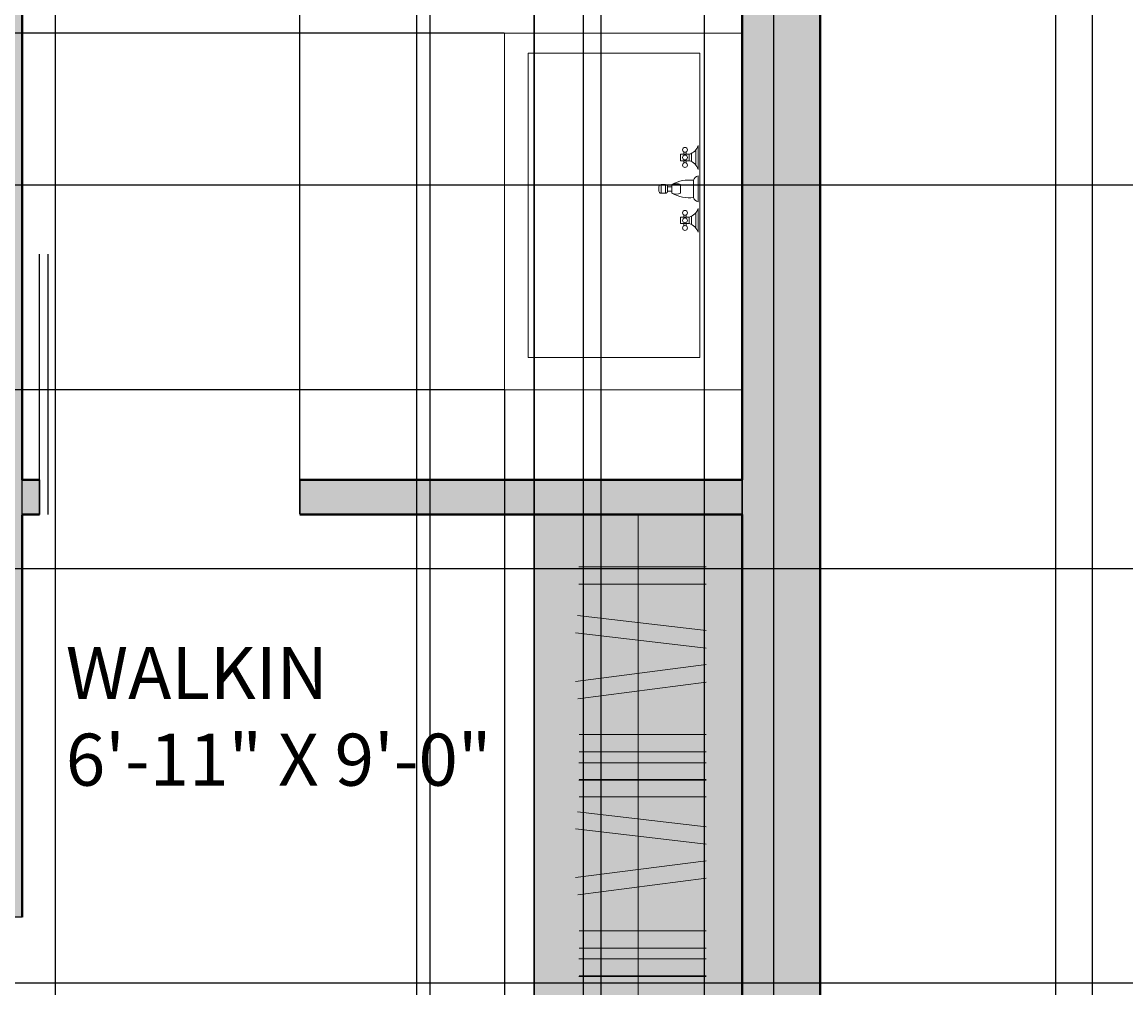
# Model space of a CAD drawing. Units: inches. Extents: x 818 to 1898, y 976 to 2364.
# Tile 44 of 96: x 1623 to 1750, y 1409 to 1520. Entities that reach past the tile are written whole.
import ezdxf

# ---------------------------------------------------------------- set-up
doc = ezdxf.new("R2010")
doc.units = ezdxf.units.IN
doc.header["$LTSCALE"] = 5
doc.header["$MEASUREMENT"] = 0
for name, color, linetype, lineweight in [('A-ANNO-DIMS', 2, 'Continuous', 18), ('A-AREA-IDEN', 7, 'Continuous', 18), ('A-DOOR', 3, 'Continuous', 25), ('A-FLOR-CASE', 8, 'Continuous', 18), ('A-FLOR-CASE-PATT', 33, 'Continuous', 9), ('A-FLOR-FIXT', 9, 'Continuous', 18), ('A-WALL', 7, 'Continuous', 40)]:
    doc.layers.add(name, color=color, linetype=linetype, lineweight=lineweight)
doc.layers.add('A-WALL-PATT', color=251, linetype='Continuous', lineweight=13, true_color=0x636466)
doc.styles.get("Standard").update_dxf_attribs({"font": 'arial.ttf'})
doc.dimstyles.get("Standard").update_dxf_attribs({"dimtxt": 0.18, "dimasz": 0.18, "dimexe": 0.18, "dimexo": 0.0625, "dimgap": 0.09, "dimtad": 0, "dimtih": 1, "dimtoh": 1, "dimdec": 4, "dimzin": 0, "dimdsep": 46, "dimtxsty": 'Standard', "dimcen": 0.09, "dimadec": 0, "dimazin": 0, "dimtfac": 1, "dimtdec": 4, "dimtofl": 0, "dimtmove": 0, "dimatfit": 3, "dimfxl": 1, "dimtolj": 1, "dimtzin": 0, "dimarcsym": 0})

# ---------------------------------------------------------------- blocks, each defined once
blk = doc.blocks.new('Faucet - Bathroom front')
for p, q in [((-0.5, 4.25), (0.5, 4.25)), ((0.5, 3.75), (-0.5, 3.75)), ((-0.5, 3), (0.5, 3)), ((-0.25, 3), (-0.25, 3.5)), ((0.25, 3.5), (0.25, 3)), ((-4, 1.625), (-4.25, 1.625)), ((-4, 1.375), (-4.25, 1.375)), ((-3.25, 1.625), (-3, 1.625)), ((-3.25, 1.375), (-3, 1.375)), ((0.5, 2), (-0.5, 2)), ((3.25, 1.625), (3, 1.625)), ((3.25, 1.375), (3, 1.375)), ((4, 1.625), (4.25, 1.625)), ((4, 1.375), (4.25, 1.375)), ((-5, 0), (-2.25, 0)), ((-4.5087, 0.25), (-2.7408, 0.25)), ((-3.1442, 0.75), (-4.0979, 0.75)), ((-1.5, 0), (1.5, 0)), ((-1, 0.5), (1, 0.5)), ((2.25, 0), (5, 0)), ((2.7413, 0.25), (4.5092, 0.25)), ((4.1058, 0.75), (3.1521, 0.75))]:
    blk.add_line(p, q)
for points in [[(-0.5, 3.75), (-0.5, 4.25)], [(-0.25, 4.5), (0.25, 4.5)], [(0.5, 4.25), (0.5, 3.75)], [(0.25, 3.5), (-0.25, 3.5)]]:
    blk.add_lwpolyline(points)
for points in [[(-4, 1), (-4, 2), (-3.25, 2), (-3.25, 1)], [(3.25, 1), (3.25, 2), (4, 2), (4, 1)]]:
    blk.add_lwpolyline(points, close=True)
for centre in [(-4.5, 1.5), (-3.625, 1.5), (-2.75, 1.5), (2.75, 1.5), (3.625, 1.5), (4.5, 1.5)]:
    blk.add_circle(centre, 0.2795)
for centre, radius, start, end in [((-0.2575, 4.2575), 0.2426, 88.22243, 181.7776), ((0.2575, 4.2575), 0.2426, 358.2224, 91.77757), ((3, 1), 4.0311, 150.2551, 187.125), ((0.6413, 2.5), 1.246, 156.3417, 203.6583), ((-0.2575, 3.7425), 0.2426, 178.2224, 271.7776), ((0.2575, 3.7425), 0.2426, 268.2224, 1.777565), ((-3, 1), 4.0311, 352.875, 29.74488), ((-0.6413, 2.5), 1.246, 336.3417, 23.65835), ((-5.375, 1.375), 1.4252, 285.2551, 344.7449), ((-1.875, 1.375), 1.4252, 195.2551, 254.7449), ((-0.7962, -0.2038), 0.7327, 106.1502, 163.8498), ((0.7962, -0.2038), 0.7327, 16.1502, 73.84979), ((1.875, 1.375), 1.4252, 285.2551, 344.7449), ((5.375, 1.375), 1.4252, 195.2551, 254.7449)]:
    blk.add_arc(centre, radius, start, end)
blk = doc.blocks.new('*D71')
at = {"layer": 'A-ANNO-DIMS', "color": 0, "lineweight": -2, "ltscale": 5, "transparency": 16777216}
for p, q in [((1714.79, 2053.08), (1897.92, 2053.08)), ((1897.74, 2052.9), (1897.74, 1699.76)), ((1897.74, 1346.26), (1897.74, 1699.4)), ((1714.79, 1346.08), (1897.92, 1346.08))]:
    blk.add_line(p, q, dxfattribs=at)
at = {"layer": 'A-ANNO-DIMS', "color": 0, "ltscale": 5, "transparency": 16777216}
for points in [[(1897.71, 2052.9), (1897.77, 2052.9), (1897.74, 2053.08)], [(1897.71, 1346.26), (1897.77, 1346.26), (1897.74, 1346.08)]]:
    blk.add_solid(points, dxfattribs=at)
at = {"layer": 'Defpoints', "color": 0, "ltscale": 5, "transparency": 16777216}
for p in [(1714.73, 2053.08), (1897.74, 2053.08), (1714.73, 1346.08)]:
    blk.add_point(p, dxfattribs=at)
at = {"layer": 'A-ANNO-DIMS', "color": 0, "ltscale": 5, "transparency": 16777216, "insert": (1897.74, 1699.58), "char_height": 0.18, "attachment_point": 5}
blk.add_mtext('\\A1;707', dxfattribs=at)
blk = doc.blocks.new('*D102')
at = {"layer": 'A-ANNO-DIMS', "color": 0, "lineweight": -2, "ltscale": 5, "transparency": 16777216}
for p, q in [((1565.48, 1071.12), (1565.48, 2363.87)), ((1626.57, 1071.12), (1626.57, 2363.87)), ((1565.66, 2363.69), (1595.63, 2363.69)), ((1626.39, 2363.69), (1596.42, 2363.69))]:
    blk.add_line(p, q, dxfattribs=at)
at = {"layer": 'A-ANNO-DIMS', "color": 0, "ltscale": 5, "transparency": 16777216}
for points in [[(1565.66, 2363.72), (1565.66, 2363.66), (1565.48, 2363.69)], [(1626.39, 2363.72), (1626.39, 2363.66), (1626.57, 2363.69)]]:
    blk.add_solid(points, dxfattribs=at)
at = {"layer": 'Defpoints', "color": 0, "ltscale": 5, "transparency": 16777216}
for p in [(1626.57, 2363.69), (1565.48, 1071.06), (1626.57, 1071.06)]:
    blk.add_point(p, dxfattribs=at)
at = {"layer": 'A-ANNO-DIMS', "color": 0, "ltscale": 5, "transparency": 16777216, "insert": (1596.03, 2363.69), "char_height": 0.18, "attachment_point": 5}
blk.add_mtext('\\A1;61.09', dxfattribs=at)
blk = doc.blocks.new('*D103')
at = {"layer": 'A-ANNO-DIMS', "color": 0, "lineweight": -2, "ltscale": 5, "transparency": 16777216}
for p, q in [((1626.57, 1071.12), (1626.57, 2363.87)), ((1689.47, 1071.12), (1689.47, 2363.87)), ((1626.75, 2363.69), (1657.7, 2363.69)), ((1689.29, 2363.69), (1658.35, 2363.69))]:
    blk.add_line(p, q, dxfattribs=at)
at = {"layer": 'A-ANNO-DIMS', "color": 0, "ltscale": 5, "transparency": 16777216}
for points in [[(1626.75, 2363.72), (1626.75, 2363.66), (1626.57, 2363.69)], [(1689.29, 2363.72), (1689.29, 2363.66), (1689.47, 2363.69)]]:
    blk.add_solid(points, dxfattribs=at)
at = {"layer": 'Defpoints', "color": 0, "ltscale": 5, "transparency": 16777216}
for p in [(1689.47, 2363.69), (1626.57, 1071.06), (1689.47, 1071.06)]:
    blk.add_point(p, dxfattribs=at)
at = {"layer": 'A-ANNO-DIMS', "color": 0, "ltscale": 5, "transparency": 16777216, "insert": (1658.02, 2363.69), "char_height": 0.18, "attachment_point": 5}
blk.add_mtext('\\A1;62.9', dxfattribs=at)
blk = doc.blocks.new('*D104')
at = {"layer": 'A-ANNO-DIMS', "color": 0, "lineweight": -2, "ltscale": 5, "transparency": 16777216}
for p, q in [((1689.47, 1071.12), (1689.47, 2363.87)), ((1746.08, 1071.12), (1746.08, 2363.87)), ((1689.65, 2363.69), (1717.4, 2363.69)), ((1745.9, 2363.69), (1718.15, 2363.69))]:
    blk.add_line(p, q, dxfattribs=at)
at = {"layer": 'A-ANNO-DIMS', "color": 0, "ltscale": 5, "transparency": 16777216}
for points in [[(1689.65, 2363.72), (1689.65, 2363.66), (1689.47, 2363.69)], [(1745.9, 2363.72), (1745.9, 2363.66), (1746.08, 2363.69)]]:
    blk.add_solid(points, dxfattribs=at)
at = {"layer": 'Defpoints', "color": 0, "ltscale": 5, "transparency": 16777216}
for p in [(1746.08, 2363.69), (1689.47, 1071.06), (1746.08, 1071.06)]:
    blk.add_point(p, dxfattribs=at)
at = {"layer": 'A-ANNO-DIMS', "color": 0, "ltscale": 5, "transparency": 16777216, "insert": (1717.78, 2363.69), "char_height": 0.18, "attachment_point": 5}
blk.add_mtext('\\A1;56.61', dxfattribs=at)
blk = doc.blocks.new('*D116')
at = {"layer": 'A-ANNO-DIMS', "color": 0, "lineweight": -2, "ltscale": 5, "transparency": 16777216}
for p, q in [((1766.29, 1456.81), (818.03, 1456.81)), ((818.21, 1456.63), (818.21, 1417.41)), ((818.21, 1377.84), (818.21, 1417.05)), ((1766.29, 1377.66), (818.03, 1377.66))]:
    blk.add_line(p, q, dxfattribs=at)
at = {"layer": 'A-ANNO-DIMS', "color": 0, "ltscale": 5, "transparency": 16777216}
for points in [[(818.18, 1456.63), (818.24, 1456.63), (818.21, 1456.81)], [(818.18, 1377.84), (818.24, 1377.84), (818.21, 1377.66)]]:
    blk.add_solid(points, dxfattribs=at)
at = {"layer": 'Defpoints', "color": 0, "ltscale": 5, "transparency": 16777216}
for p in [(818.21, 1456.81), (1766.35, 1456.81), (1766.35, 1377.66)]:
    blk.add_point(p, dxfattribs=at)
at = {"layer": 'A-ANNO-DIMS', "color": 0, "ltscale": 5, "transparency": 16777216, "insert": (818.21, 1417.23), "char_height": 0.18, "attachment_point": 5}
blk.add_mtext('\\A1;79.15', dxfattribs=at)
blk = doc.blocks.new('*D117')
at = {"layer": 'A-ANNO-DIMS', "color": 0, "lineweight": -2, "ltscale": 5, "transparency": 16777216}
for p, q in [((1766.29, 1545.18), (818.03, 1545.18)), ((818.21, 1545), (818.21, 1501.18)), ((818.21, 1456.99), (818.21, 1500.81)), ((1766.29, 1456.81), (818.03, 1456.81))]:
    blk.add_line(p, q, dxfattribs=at)
at = {"layer": 'A-ANNO-DIMS', "color": 0, "ltscale": 5, "transparency": 16777216}
for points in [[(818.18, 1545), (818.24, 1545), (818.21, 1545.18)], [(818.18, 1456.99), (818.24, 1456.99), (818.21, 1456.81)]]:
    blk.add_solid(points, dxfattribs=at)
at = {"layer": 'Defpoints', "color": 0, "ltscale": 5, "transparency": 16777216}
for p in [(818.21, 1545.18), (1766.35, 1545.18), (1766.35, 1456.81)]:
    blk.add_point(p, dxfattribs=at)
at = {"layer": 'A-ANNO-DIMS', "color": 0, "ltscale": 5, "transparency": 16777216, "insert": (818.21, 1501), "char_height": 0.18, "attachment_point": 5}
blk.add_mtext('\\A1;88.37', dxfattribs=at)
blk = doc.blocks.new('*D154')
at = {"layer": 'A-ANNO-DIMS', "color": 0, "lineweight": -2, "ltscale": 5, "transparency": 16777216}
for p, q in [((1701.37, 1290.14), (1701.37, 2363.87)), ((1709.37, 1298.14), (1709.37, 2363.87)), ((1701.55, 2363.69), (1705.22, 2363.69)), ((1709.19, 2363.69), (1705.52, 2363.69))]:
    blk.add_line(p, q, dxfattribs=at)
at = {"layer": 'A-ANNO-DIMS', "color": 0, "ltscale": 5, "transparency": 16777216}
for points in [[(1701.55, 2363.72), (1701.55, 2363.66), (1701.37, 2363.69)], [(1709.19, 2363.72), (1709.19, 2363.66), (1709.37, 2363.69)]]:
    blk.add_solid(points, dxfattribs=at)
at = {"layer": 'Defpoints', "color": 0, "ltscale": 5, "transparency": 16777216}
for p in [(1709.37, 2363.69), (1709.37, 1298.08), (1701.37, 1290.08)]:
    blk.add_point(p, dxfattribs=at)
at = {"layer": 'A-ANNO-DIMS', "color": 0, "ltscale": 5, "transparency": 16777216, "insert": (1705.37, 2363.69), "char_height": 0.18, "attachment_point": 5}
blk.add_mtext('\\A1;8', dxfattribs=at)
blk = doc.blocks.new('*D170')
at = {"layer": 'A-ANNO-DIMS', "color": 0, "lineweight": -2, "ltscale": 5, "transparency": 16777216}
for p, q in [((1430.79, 1600.08), (1897.92, 1600.08)), ((1897.74, 1599.9), (1897.74, 1550.76)), ((1897.74, 1501.26), (1897.74, 1550.4)), ((1430.79, 1501.08), (1897.92, 1501.08))]:
    blk.add_line(p, q, dxfattribs=at)
at = {"layer": 'A-ANNO-DIMS', "color": 0, "ltscale": 5, "transparency": 16777216}
for points in [[(1897.71, 1599.9), (1897.77, 1599.9), (1897.74, 1600.08)], [(1897.71, 1501.26), (1897.77, 1501.26), (1897.74, 1501.08)]]:
    blk.add_solid(points, dxfattribs=at)
at = {"layer": 'Defpoints', "color": 0, "ltscale": 5, "transparency": 16777216}
for p in [(1430.73, 1600.08), (1897.74, 1600.08), (1430.73, 1501.08)]:
    blk.add_point(p, dxfattribs=at)
at = {"layer": 'A-ANNO-DIMS', "color": 0, "ltscale": 5, "transparency": 16777216, "insert": (1897.74, 1550.58), "char_height": 0.18, "attachment_point": 5}
blk.add_mtext('\\A1;99', dxfattribs=at)
blk = doc.blocks.new('*D173')
at = {"layer": 'A-ANNO-DIMS', "color": 0, "lineweight": -2, "ltscale": 5, "transparency": 16777216}
for p, q in [((1622.73, 1463.14), (1622.73, 2363.87)), ((1654.73, 1463.14), (1654.73, 2363.87)), ((1622.91, 2363.69), (1638.51, 2363.69)), ((1654.55, 2363.69), (1638.94, 2363.69))]:
    blk.add_line(p, q, dxfattribs=at)
at = {"layer": 'A-ANNO-DIMS', "color": 0, "ltscale": 5, "transparency": 16777216}
for points in [[(1622.91, 2363.72), (1622.91, 2363.66), (1622.73, 2363.69)], [(1654.55, 2363.72), (1654.55, 2363.66), (1654.73, 2363.69)]]:
    blk.add_solid(points, dxfattribs=at)
at = {"layer": 'Defpoints', "color": 0, "ltscale": 5, "transparency": 16777216}
for p in [(1654.73, 2363.69), (1622.73, 1463.08), (1654.73, 1463.08)]:
    blk.add_point(p, dxfattribs=at)
at = {"layer": 'A-ANNO-DIMS', "color": 0, "ltscale": 5, "transparency": 16777216, "insert": (1638.73, 2363.69), "char_height": 0.18, "attachment_point": 5}
blk.add_mtext('\\A1;32', dxfattribs=at)
blk = doc.blocks.new('*D178')
at = {"layer": 'A-ANNO-DIMS', "color": 0, "lineweight": -2, "ltscale": 5, "transparency": 16777216}
for p, q in [((1669.73, 1600.02), (1669.73, 975.66)), ((1705.73, 1600.02), (1705.73, 975.66)), ((1669.91, 975.84), (1687.51, 975.84)), ((1705.55, 975.84), (1687.94, 975.84))]:
    blk.add_line(p, q, dxfattribs=at)
at = {"layer": 'A-ANNO-DIMS', "color": 0, "ltscale": 5, "transparency": 16777216}
for points in [[(1669.91, 975.87), (1669.91, 975.81), (1669.73, 975.84)], [(1705.55, 975.87), (1705.55, 975.81), (1705.73, 975.84)]]:
    blk.add_solid(points, dxfattribs=at)
at = {"layer": 'Defpoints', "color": 0, "ltscale": 5, "transparency": 16777216}
for p in [(1669.73, 1600.08), (1705.73, 1600.08), (1705.73, 975.84)]:
    blk.add_point(p, dxfattribs=at)
at = {"layer": 'A-ANNO-DIMS', "color": 0, "ltscale": 5, "transparency": 16777216, "insert": (1687.73, 975.84), "char_height": 0.18, "attachment_point": 5}
blk.add_mtext('\\A1;36', dxfattribs=at)
blk = doc.blocks.new('*D180')
at = {"layer": 'A-ANNO-DIMS', "color": 0, "lineweight": -2, "ltscale": 5, "transparency": 16777216}
for p, q in [((1599.73, 1639.52), (1599.73, 975.66)), ((1669.73, 1639.52), (1669.73, 975.66)), ((1599.91, 975.84), (1634.51, 975.84)), ((1669.55, 975.84), (1634.94, 975.84))]:
    blk.add_line(p, q, dxfattribs=at)
at = {"layer": 'A-ANNO-DIMS', "color": 0, "ltscale": 5, "transparency": 16777216}
for points in [[(1599.91, 975.87), (1599.91, 975.81), (1599.73, 975.84)], [(1669.55, 975.87), (1669.55, 975.81), (1669.73, 975.84)]]:
    blk.add_solid(points, dxfattribs=at)
at = {"layer": 'Defpoints', "color": 0, "ltscale": 5, "transparency": 16777216}
for p in [(1599.73, 1639.58), (1669.73, 1639.58), (1669.73, 975.84)]:
    blk.add_point(p, dxfattribs=at)
at = {"layer": 'A-ANNO-DIMS', "color": 0, "ltscale": 5, "transparency": 16777216, "insert": (1634.73, 975.84), "char_height": 0.18, "attachment_point": 5}
blk.add_mtext('\\A1;70', dxfattribs=at)
blk = doc.blocks.new('*D183')
at = {"layer": 'A-ANNO-DIMS', "color": 0, "lineweight": -2, "ltscale": 5, "transparency": 16777216}
for p, q in [((1714.73, 1545.02), (1714.73, 975.66)), ((1741.84, 1545.02), (1741.84, 975.66)), ((1714.91, 975.84), (1727.82, 975.84)), ((1741.66, 975.84), (1728.75, 975.84))]:
    blk.add_line(p, q, dxfattribs=at)
at = {"layer": 'A-ANNO-DIMS', "color": 0, "ltscale": 5, "transparency": 16777216}
for points in [[(1714.91, 975.87), (1714.91, 975.81), (1714.73, 975.84)], [(1741.66, 975.87), (1741.66, 975.81), (1741.84, 975.84)]]:
    blk.add_solid(points, dxfattribs=at)
at = {"layer": 'Defpoints', "color": 0, "ltscale": 5, "transparency": 16777216}
for p in [(1714.73, 1545.08), (1741.84, 1545.08), (1741.84, 975.84)]:
    blk.add_point(p, dxfattribs=at)
at = {"layer": 'A-ANNO-DIMS', "color": 0, "ltscale": 5, "transparency": 16777216, "insert": (1728.28, 975.84), "char_height": 0.18, "attachment_point": 5}
blk.add_mtext('\\A1;27.116', dxfattribs=at)
blk = doc.blocks.new('*D188')
at = {"layer": 'A-ANNO-DIMS', "color": 0, "lineweight": -2, "ltscale": 5, "transparency": 16777216}
for p, q in [((1714.79, 1545.08), (1897.92, 1545.08)), ((1897.74, 1544.9), (1897.74, 1445.76)), ((1897.74, 1346.26), (1897.74, 1445.4)), ((1714.79, 1346.08), (1897.92, 1346.08))]:
    blk.add_line(p, q, dxfattribs=at)
at = {"layer": 'A-ANNO-DIMS', "color": 0, "ltscale": 5, "transparency": 16777216}
for points in [[(1897.71, 1544.9), (1897.77, 1544.9), (1897.74, 1545.08)], [(1897.71, 1346.26), (1897.77, 1346.26), (1897.74, 1346.08)]]:
    blk.add_solid(points, dxfattribs=at)
at = {"layer": 'Defpoints', "color": 0, "ltscale": 5, "transparency": 16777216}
for p in [(1714.73, 1545.08), (1897.74, 1545.08), (1714.73, 1346.08)]:
    blk.add_point(p, dxfattribs=at)
at = {"layer": 'A-ANNO-DIMS', "color": 0, "ltscale": 5, "transparency": 16777216, "insert": (1897.74, 1445.58), "char_height": 0.18, "attachment_point": 5}
blk.add_mtext('\\A1;199', dxfattribs=at)
blk = doc.blocks.new('*D195')
at = {"layer": 'A-ANNO-DIMS', "color": 0, "lineweight": -2, "ltscale": 5, "transparency": 16777216}
for p, q in [((1681.73, 1379.14), (1681.73, 2363.87)), ((1705.73, 1355.14), (1705.73, 2363.87)), ((1681.91, 2363.69), (1693.51, 2363.69)), ((1705.55, 2363.69), (1693.95, 2363.69))]:
    blk.add_line(p, q, dxfattribs=at)
at = {"layer": 'A-ANNO-DIMS', "color": 0, "ltscale": 5, "transparency": 16777216}
for points in [[(1681.91, 2363.72), (1681.91, 2363.66), (1681.73, 2363.69)], [(1705.55, 2363.72), (1705.55, 2363.66), (1705.73, 2363.69)]]:
    blk.add_solid(points, dxfattribs=at)
at = {"layer": 'Defpoints', "color": 0, "ltscale": 5, "transparency": 16777216}
for p in [(1705.73, 2363.69), (1681.73, 1379.08), (1705.73, 1355.08)]:
    blk.add_point(p, dxfattribs=at)
at = {"layer": 'A-ANNO-DIMS', "color": 0, "ltscale": 5, "transparency": 16777216, "insert": (1693.73, 2363.69), "char_height": 0.18, "attachment_point": 5}
blk.add_mtext('\\A1;24', dxfattribs=at)
blk = doc.blocks.new('*D197')
at = {"layer": 'A-ANNO-DIMS', "color": 0, "lineweight": -2, "ltscale": 5, "transparency": 16777216}
for p, q in [((1457.79, 1526.67), (1897.92, 1526.67)), ((1897.74, 1526.49), (1897.74, 1468.08)), ((1897.74, 1409.3), (1897.74, 1467.71)), ((1457.79, 1409.12), (1897.92, 1409.12))]:
    blk.add_line(p, q, dxfattribs=at)
at = {"layer": 'A-ANNO-DIMS', "color": 0, "ltscale": 5, "transparency": 16777216}
for points in [[(1897.71, 1526.49), (1897.77, 1526.49), (1897.74, 1526.67)], [(1897.71, 1409.3), (1897.77, 1409.3), (1897.74, 1409.12)]]:
    blk.add_solid(points, dxfattribs=at)
at = {"layer": 'Defpoints', "color": 0, "ltscale": 5, "transparency": 16777216}
for p in [(1457.73, 1526.67), (1897.74, 1526.67), (1457.73, 1409.12)]:
    blk.add_point(p, dxfattribs=at)
at = {"layer": 'A-ANNO-DIMS', "color": 0, "ltscale": 5, "transparency": 16777216, "insert": (1897.74, 1467.89), "char_height": 0.18, "attachment_point": 5}
blk.add_mtext('\\A1;117.55', dxfattribs=at)
blk = doc.blocks.new('*D198')
at = {"layer": 'A-ANNO-DIMS', "color": 0, "lineweight": -2, "ltscale": 5, "transparency": 16777216}
for p, q in [((1741.84, 1545.02), (1741.84, 975.66)), ((1430.73, 1346.02), (1430.73, 975.66)), ((1430.91, 975.84), (1585.91, 975.84)), ((1741.66, 975.84), (1586.66, 975.84))]:
    blk.add_line(p, q, dxfattribs=at)
at = {"layer": 'A-ANNO-DIMS', "color": 0, "ltscale": 5, "transparency": 16777216}
for points in [[(1430.91, 975.87), (1430.91, 975.81), (1430.73, 975.84)], [(1741.66, 975.87), (1741.66, 975.81), (1741.84, 975.84)]]:
    blk.add_solid(points, dxfattribs=at)
at = {"layer": 'Defpoints', "color": 0, "ltscale": 5, "transparency": 16777216}
for p in [(1741.84, 1545.08), (1430.73, 1346.08), (1741.84, 975.84)]:
    blk.add_point(p, dxfattribs=at)
at = {"layer": 'A-ANNO-DIMS', "color": 0, "ltscale": 5, "transparency": 16777216, "insert": (1586.28, 975.84), "char_height": 0.18, "attachment_point": 5}
blk.add_mtext('\\A1;311.1', dxfattribs=at)
blk = doc.blocks.new('*D199')
at = {"layer": 'A-ANNO-DIMS', "color": 0, "lineweight": -2, "ltscale": 5, "transparency": 16777216}
for p, q in [((1559.79, 1687.08), (1897.92, 1687.08)), ((1897.74, 1686.9), (1897.74, 1513.15)), ((1897.74, 1339.05), (1897.74, 1512.79)), ((1660.38, 1338.87), (1897.92, 1338.87))]:
    blk.add_line(p, q, dxfattribs=at)
at = {"layer": 'A-ANNO-DIMS', "color": 0, "ltscale": 5, "transparency": 16777216}
for points in [[(1897.71, 1686.9), (1897.77, 1686.9), (1897.74, 1687.08)], [(1897.71, 1339.05), (1897.77, 1339.05), (1897.74, 1338.87)]]:
    blk.add_solid(points, dxfattribs=at)
at = {"layer": 'Defpoints', "color": 0, "ltscale": 5, "transparency": 16777216}
for p in [(1559.73, 1687.08), (1897.74, 1687.08), (1660.31, 1338.87)]:
    blk.add_point(p, dxfattribs=at)
at = {"layer": 'A-ANNO-DIMS', "color": 0, "ltscale": 5, "transparency": 16777216, "insert": (1897.74, 1512.97), "char_height": 0.18, "attachment_point": 5}
blk.add_mtext('\\A1;348.2', dxfattribs=at)
blk = doc.blocks.new('*D200')
at = {"layer": 'A-ANNO-DIMS', "color": 0, "lineweight": -2, "ltscale": 5, "transparency": 16777216}
for p, q in [((1678.33, 1477.36), (1678.33, 975.66)), ((1705.73, 1477.36), (1705.73, 975.66)), ((1678.51, 975.84), (1691.56, 975.84)), ((1705.55, 975.84), (1692.49, 975.84))]:
    blk.add_line(p, q, dxfattribs=at)
at = {"layer": 'A-ANNO-DIMS', "color": 0, "ltscale": 5, "transparency": 16777216}
for points in [[(1678.51, 975.87), (1678.51, 975.81), (1678.33, 975.84)], [(1705.55, 975.87), (1705.55, 975.81), (1705.73, 975.84)]]:
    blk.add_solid(points, dxfattribs=at)
at = {"layer": 'Defpoints', "color": 0, "ltscale": 5, "transparency": 16777216}
for p in [(1678.33, 1477.43), (1705.73, 1477.43), (1705.73, 975.84)]:
    blk.add_point(p, dxfattribs=at)
at = {"layer": 'A-ANNO-DIMS', "color": 0, "ltscale": 5, "transparency": 16777216, "insert": (1692.03, 975.84), "char_height": 0.18, "attachment_point": 5}
blk.add_mtext('\\A1;27.395', dxfattribs=at)
blk = doc.blocks.new('*D201')
at = {"layer": 'A-ANNO-DIMS', "color": 0, "lineweight": -2, "ltscale": 5, "transparency": 16777216}
for p, q in [((1678.27, 1518.56), (818.03, 1518.56)), ((818.21, 1518.38), (818.21, 1498.18)), ((818.21, 1477.61), (818.21, 1497.81)), ((1678.27, 1477.43), (818.03, 1477.43))]:
    blk.add_line(p, q, dxfattribs=at)
at = {"layer": 'A-ANNO-DIMS', "color": 0, "ltscale": 5, "transparency": 16777216}
for points in [[(818.18, 1518.38), (818.24, 1518.38), (818.21, 1518.56)], [(818.18, 1477.61), (818.24, 1477.61), (818.21, 1477.43)]]:
    blk.add_solid(points, dxfattribs=at)
at = {"layer": 'Defpoints', "color": 0, "ltscale": 5, "transparency": 16777216}
for p in [(818.21, 1518.56), (1678.33, 1518.56), (1678.33, 1477.43)]:
    blk.add_point(p, dxfattribs=at)
at = {"layer": 'A-ANNO-DIMS', "color": 0, "ltscale": 5, "transparency": 16777216, "insert": (818.21, 1497.99), "char_height": 0.18, "attachment_point": 5}
blk.add_mtext('\\A1;41.135', dxfattribs=at)
blk = doc.blocks.new('*D212')
at = {"layer": 'A-ANNO-DIMS', "color": 0, "lineweight": -2, "ltscale": 5, "transparency": 16777216}
for p, q in [((1681.73, 1900.02), (1681.73, 975.66)), ((1705.73, 1876.02), (1705.73, 975.66)), ((1681.91, 975.84), (1693.51, 975.84)), ((1705.55, 975.84), (1693.95, 975.84))]:
    blk.add_line(p, q, dxfattribs=at)
at = {"layer": 'A-ANNO-DIMS', "color": 0, "ltscale": 5, "transparency": 16777216}
for points in [[(1681.91, 975.87), (1681.91, 975.81), (1681.73, 975.84)], [(1705.55, 975.87), (1705.55, 975.81), (1705.73, 975.84)]]:
    blk.add_solid(points, dxfattribs=at)
at = {"layer": 'Defpoints', "color": 0, "ltscale": 5, "transparency": 16777216}
for p in [(1681.73, 1900.08), (1705.73, 1876.08), (1705.73, 975.84)]:
    blk.add_point(p, dxfattribs=at)
at = {"layer": 'A-ANNO-DIMS', "color": 0, "ltscale": 5, "transparency": 16777216, "insert": (1693.73, 975.84), "char_height": 0.18, "attachment_point": 5}
blk.add_mtext('\\A1;24', dxfattribs=at)
blk = doc.blocks.new('*D214')
at = {"layer": 'A-ANNO-DIMS', "color": 0, "lineweight": -2, "ltscale": 5, "transparency": 16777216}
for p, q in [((1511.73, 1687.02), (1511.73, 975.66)), ((1714.73, 1687.02), (1714.73, 975.66)), ((1511.91, 975.84), (1612.93, 975.84)), ((1714.55, 975.84), (1613.52, 975.84))]:
    blk.add_line(p, q, dxfattribs=at)
at = {"layer": 'A-ANNO-DIMS', "color": 0, "ltscale": 5, "transparency": 16777216}
for points in [[(1511.91, 975.87), (1511.91, 975.81), (1511.73, 975.84)], [(1714.55, 975.87), (1714.55, 975.81), (1714.73, 975.84)]]:
    blk.add_solid(points, dxfattribs=at)
at = {"layer": 'Defpoints', "color": 0, "ltscale": 5, "transparency": 16777216}
for p in [(1511.73, 1687.08), (1714.73, 1687.08), (1714.73, 975.84)]:
    blk.add_point(p, dxfattribs=at)
at = {"layer": 'A-ANNO-DIMS', "color": 0, "ltscale": 5, "transparency": 16777216, "insert": (1613.23, 975.84), "char_height": 0.18, "attachment_point": 5}
blk.add_mtext('\\A1;203', dxfattribs=at)
blk = doc.blocks.new('*D221')
at = {"layer": 'A-ANNO-DIMS', "color": 0, "lineweight": -2, "ltscale": 5, "transparency": 16777216}
for p, q in [((1668.18, 1696.02), (1668.18, 975.66)), ((1705.73, 1696.02), (1705.73, 975.66)), ((1668.36, 975.84), (1686.56, 975.84)), ((1705.55, 975.84), (1687.35, 975.84))]:
    blk.add_line(p, q, dxfattribs=at)
at = {"layer": 'A-ANNO-DIMS', "color": 0, "ltscale": 5, "transparency": 16777216}
for points in [[(1668.36, 975.87), (1668.36, 975.81), (1668.18, 975.84)], [(1705.55, 975.87), (1705.55, 975.81), (1705.73, 975.84)]]:
    blk.add_solid(points, dxfattribs=at)
at = {"layer": 'Defpoints', "color": 0, "ltscale": 5, "transparency": 16777216}
for p in [(1668.18, 1696.08), (1705.73, 1696.08), (1705.73, 975.84)]:
    blk.add_point(p, dxfattribs=at)
at = {"layer": 'A-ANNO-DIMS', "color": 0, "ltscale": 5, "transparency": 16777216, "insert": (1686.95, 975.84), "char_height": 0.18, "attachment_point": 5}
blk.add_mtext('\\A1;37.54', dxfattribs=at)
blk = doc.blocks.new('*D228')
at = {"layer": 'A-ANNO-DIMS', "color": 0, "lineweight": -2, "ltscale": 5, "transparency": 16777216}
for p, q in [((1687.39, 1802.02), (1687.39, 975.66)), ((1705.73, 1802.02), (1705.73, 975.66)), ((1687.57, 975.84), (1696.17, 975.84)), ((1705.55, 975.84), (1696.94, 975.84))]:
    blk.add_line(p, q, dxfattribs=at)
at = {"layer": 'A-ANNO-DIMS', "color": 0, "ltscale": 5, "transparency": 16777216}
for points in [[(1687.57, 975.87), (1687.57, 975.81), (1687.39, 975.84)], [(1705.55, 975.87), (1705.55, 975.81), (1705.73, 975.84)]]:
    blk.add_solid(points, dxfattribs=at)
at = {"layer": 'Defpoints', "color": 0, "ltscale": 5, "transparency": 16777216}
for p in [(1687.39, 1802.08), (1705.73, 1802.08), (1705.73, 975.84)]:
    blk.add_point(p, dxfattribs=at)
at = {"layer": 'A-ANNO-DIMS', "color": 0, "ltscale": 5, "transparency": 16777216, "insert": (1696.56, 975.84), "char_height": 0.18, "attachment_point": 5}
blk.add_mtext('\\A1;18.33', dxfattribs=at)
blk = doc.blocks.new('*D267')
at = {"layer": 'A-ANNO-DIMS', "color": 0, "lineweight": -2, "ltscale": 5, "transparency": 16777216}
for p, q in [((1714.73, 1687.02), (1714.73, 975.66)), ((1741.84, 1687.02), (1741.84, 975.66)), ((1714.91, 975.84), (1727.82, 975.84)), ((1741.66, 975.84), (1728.75, 975.84))]:
    blk.add_line(p, q, dxfattribs=at)
at = {"layer": 'A-ANNO-DIMS', "color": 0, "ltscale": 5, "transparency": 16777216}
for points in [[(1714.91, 975.87), (1714.91, 975.81), (1714.73, 975.84)], [(1741.66, 975.87), (1741.66, 975.81), (1741.84, 975.84)]]:
    blk.add_solid(points, dxfattribs=at)
at = {"layer": 'Defpoints', "color": 0, "ltscale": 5, "transparency": 16777216}
for p in [(1714.73, 1687.08), (1741.84, 1687.08), (1741.84, 975.84)]:
    blk.add_point(p, dxfattribs=at)
at = {"layer": 'A-ANNO-DIMS', "color": 0, "ltscale": 5, "transparency": 16777216, "insert": (1728.28, 975.84), "char_height": 0.18, "attachment_point": 5}
blk.add_mtext('\\A1;27.116', dxfattribs=at)

msp = doc.modelspace()

# ---------------------------------------------------------------- hatches: boundary and pattern name
at = {"layer": 'A-FLOR-CASE-PATT', "ltscale": 5}
h = msp.add_hatch(color=256, dxfattribs=at)
h.dxf.hatch_style = 1
h.paths.add_polyline_path([(1705.7251, 1941.0782), (1681.7251, 1941.0782), (1681.7251, 1900.0782), (1599.7251, 1900.0782), (1599.7251, 1876.0782), (1705.7251, 1876.0782)])
h.paths.add_polyline_path([(1457.7251, 1409.1177), (1457.7251, 1526.6712), (1439.7252, 1526.6712), (1439.7252, 1457.5313), (1446.3307, 1457.5313), (1446.3307, 1468.9514), (1446.8307, 1470.665), (1446.8307, 1469.665), (1446.8307, 1468.9514), (1446.8307, 1456.8361), (1446.8307, 1444.7258), (1446.8307, 1443.3338), (1446.3307, 1444.7258), (1446.3307, 1456.8361), (1439.7252, 1456.8361), (1439.7252, 1355.0782), (1463.7252, 1355.0782), (1463.7252, 1367.3287), (1458.0475, 1367.3287, -0.23606798), (1457.0475, 1369.3287), (1456.0475, 1369.3287, -0.11764706), (1456.0475, 1386.3287), (1457.0475, 1386.3287, -0.23606798), (1458.0475, 1388.3287), (1463.7252, 1388.3287), (1463.7252, 1389.3211)])
h.paths.add_polyline_path([(1341.2593, 1534.0782), (1246.9377, 1534.0782), (1246.9377, 1510.0782), (1341.2593, 1510.0782)])
h.paths.add_polyline_path([(1288.8272, 1519.927), (1289.8272, 1519.927), (1290.5408, 1519.927), (1302.6561, 1519.927), (1314.7664, 1519.927), (1316.1584, 1519.927), (1314.7664, 1519.427), (1302.6561, 1519.427), (1302.6561, 1512.8214), (1301.9609, 1512.8214), (1301.9609, 1519.427), (1290.5408, 1519.427)], flags=16)
h.paths.add_polyline_path([(1377.7791, 1867.0782), (1344.5531, 1867.0782), (1344.5531, 1860.4726), (1355.9731, 1860.4726), (1357.6867, 1859.9726), (1356.6867, 1859.9726), (1355.9731, 1859.9726), (1343.8579, 1859.9726), (1331.7475, 1859.9726), (1330.3556, 1859.9726), (1331.7475, 1860.4726), (1343.8579, 1860.4726), (1343.8579, 1867.0782), (1311.3271, 1867.0782), (1311.3271, 1853.7496), (1377.7791, 1853.7496)])
h.paths.add_polyline_path([(1301.148, 1610.7299, -0.46196039), (1314.4882, 1599.3725, -0.19222541), (1311.3254, 1591.4497, 0.54791519), (1336.8832, 1607.7707, 0.92061359)])
h.paths.add_polyline_path([(1370.719, 1780.5695, 1), (1332.478, 1780.5695, 1)])
h.paths.add_polyline_path([(1705.7251, 1463.0782), (1681.7251, 1463.0782), (1681.7251, 1379.0782), (1622.7251, 1379.0782), (1622.7251, 1355.0782), (1705.7251, 1355.0782)])
h.paths.add_polyline_path([(1658.1052, 1359.2188), (1658.1786, 1359.2188), (1658.1786, 1373.8763), (1658.1052, 1373.9202)], flags=16)
h.paths.add_polyline_path([(1686.9271, 1409.9311), (1686.8832, 1409.8578), (1701.5845, 1409.8578), (1701.5845, 1409.9311)], flags=16)
h.paths.add_polyline_path([(1637.1266, 1359.2188), (1637.2, 1359.2188), (1637.2, 1373.8763), (1637.1266, 1373.9202)], flags=16)
at = {"layer": 'A-WALL-PATT', "ltscale": 5}
h = msp.add_hatch(color=256, dxfattribs=at)
h.dxf.hatch_style = 1
h.paths.add_polyline_path([(1267.7252, 1928.9218), (1258.7252, 1928.9218), (1258.7252, 1913.6401), (1250.3029, 1913.6401), (1250.3029, 1878.3919), (1258.7252, 1878.3919), (1258.7252, 1862.9652), (1267.7252, 1862.9652)])
h.paths.add_polyline_path([(1267.7252, 1814.9652), (1258.7252, 1814.9652), (1258.7252, 1755.3321), (1267.7252, 1755.3321)])
h.paths.add_polyline_path([(1463.7252, 1696.0782), (1267.7252, 1696.0782), (1267.7252, 1707.3321), (1258.7252, 1707.3321), (1258.7252, 1700.0782), (1251.9333, 1700.0782), (1251.9333, 1687.0782), (1463.7252, 1687.0782)])
h.paths.add_polyline_path([(1714.7251, 1717.3178), (1705.7251, 1717.3178), (1705.7251, 1696.0782), (1599.7251, 1696.0782), (1599.7251, 1790.0782), (1705.7251, 1790.0782), (1705.7251, 1785.6125), (1714.7251, 1785.6125), (1714.7251, 1827.2125), (1705.7251, 1827.2125), (1705.7251, 1802.0782), (1599.7251, 1802.0782), (1599.7251, 1867.0782), (1705.7251, 1867.0782), (1705.7251, 1857.2125), (1714.7251, 1857.2125), (1714.7251, 1930.0316), (1741.8409, 1930.0316), (1741.8409, 1935.0316), (1714.7251, 1935.0316), (1714.7251, 1957.0338), (1741.8409, 1957.0338), (1741.8409, 1962.0338), (1714.7251, 1962.0338), (1705.7251, 1962.0338), (1705.7251, 1948.0782), (1599.7251, 1948.0782), (1599.7251, 1981.0782), (1590.7252, 1981.0782), (1590.7252, 1941.0782), (1620.7252, 1941.0782), (1705.7251, 1941.0782), (1705.7251, 1876.0782), (1599.7251, 1876.0782), (1599.7251, 1911.0782), (1590.7252, 1911.0782), (1590.7252, 1876.0782), (1429.2252, 1876.0782), (1429.2252, 1867.0782), (1511.7251, 1867.0782), (1528.593, 1867.0782), (1595.7252, 1867.0782), (1595.7252, 1773.0782), (1520.7252, 1773.0782), (1520.7252, 1837.5823), (1532.593, 1837.5823), (1532.593, 1867.0782), (1528.593, 1867.0782), (1528.593, 1841.5823), (1511.7251, 1841.5823), (1511.7251, 1744.9714), (1520.7252, 1744.9714), (1520.7252, 1761.0782), (1595.7252, 1761.0782), (1595.7252, 1696.0782), (1520.7252, 1696.0782), (1520.7252, 1716.0454), (1511.7251, 1716.0454), (1511.7251, 1696.0782), (1511.7251, 1687.0782), (1714.7251, 1687.0782)])
h.paths.add_polyline_path([(1714.7251, 2053.0782), (1714.7251, 2081.1881), (1709.7252, 2081.1881), (1709.7252, 2053.0782), (1681.6446, 2053.0782), (1681.6446, 2081.1881), (1676.6446, 2081.1881), (1676.6446, 2053.0782), (1538.5155, 2053.0782), (1538.5155, 2044.0782), (1590.7252, 2044.0782), (1590.7252, 2011.0782), (1599.7251, 2011.0782), (1599.7251, 2044.0782), (1705.7251, 2044.0782), (1705.7251, 2014.5114), (1714.7251, 2014.5114)])
h.paths.add_polyline_path([(1485.1216, 2053.0782), (1422.02, 2053.0782), (1422.02, 2081.1881), (1413.02, 2081.1881), (1413.02, 2053.0782), (1399.6356, 2053.0782), (1399.6356, 2081.1881), (1390.6356, 2081.1881), (1390.6356, 2053.0782), (1388.0315, 2053.0782), (1388.0315, 2044.0782), (1416.2743, 2044.0782), (1485.1216, 2044.0782)])
h.paths.add_polyline_path([(1330.305, 2053.0782), (1258.7252, 2053.0782), (1258.7252, 2019.2871), (1267.7252, 2019.2871), (1267.7252, 2044.0782), (1330.305, 2044.0782)])
h.paths.add_polyline_path([(1258.7252, 2053.0782), (1214.6577, 2053.0782), (1214.6577, 2044.0782), (1258.7252, 2044.0782)])
h.paths.add_polyline_path([(1214.6577, 2053.0782), (1180.349, 2053.0782), (1180.349, 2044.0782), (1214.6577, 2044.0782)])
h.paths.add_polyline_path([(1714.7251, 1639.5782), (1741.8409, 1639.5782), (1741.8409, 1643.5782), (1714.7251, 1643.5782), (1714.7251, 1649.9029), (1705.7251, 1649.9029), (1705.7251, 1600.0782), (1477.7252, 1600.0782), (1477.7252, 1591.0782), (1520.7252, 1591.0782), (1616.7252, 1591.0782), (1616.7252, 1416.6857), (1622.7251, 1416.6857), (1622.7251, 1463.0782), (1624.7252, 1463.0782), (1624.7252, 1467.0782), (1622.7251, 1467.0782), (1622.7251, 1591.0782), (1705.7251, 1591.0782), (1705.7251, 1545.0782), (1714.7251, 1545.0782), (1741.8409, 1545.0782), (1741.8409, 1549.0782), (1714.7251, 1549.0782), (1714.7251, 1593.9175), (1737.8409, 1593.9175), (1737.8409, 1597.9175), (1714.7251, 1597.9175)])
h.paths.add_polyline_path([(1674.9024, 2060.7419), (1714.7045, 2060.7419), (1714.7045, 2073.1061), (1674.9024, 2073.1061)], flags=25)
h.paths.add_polyline_path([(1394.5468, 2061.6618), (1422.2344, 2061.6618), (1422.2344, 2074.0261), (1394.5468, 2074.0261)], flags=24)
h = msp.add_hatch(color=256, dxfattribs=at)
h.dxf.hatch_style = 1
h.paths.add_polyline_path([(1714.7251, 1521.0782), (1705.7251, 1521.0782), (1705.7251, 1467.0782), (1654.7251, 1467.0782), (1654.7251, 1463.0782), (1705.7251, 1463.0782), (1705.7251, 1355.0782), (1622.7251, 1355.0782), (1622.7251, 1379.0782), (1622.7251, 1386.6857), (1616.7252, 1386.6857), (1616.7252, 1355.0782), (1490.9163, 1355.0782), (1490.9163, 1346.0782), (1544.7605, 1346.0782), (1544.6132, 1346.8783), (1544.6729, 1346.84), (1544.6299, 1346.7874), (1544.7605, 1346.0782), (1555.1299, 1346.0782), (1555.1299, 1341.5528), (1556.1599, 1340.8639), (1556.5281, 1338.8654), (1660.3141, 1338.8654), (1660.3141, 1346.0782), (1705.7251, 1346.0782), (1705.7251, 1345.0768), (1705.8704, 1344.58), (1705.7251, 1344.3933), (1705.7251, 1334.9904), (1705.8704, 1334.4936), (1705.7251, 1334.3068), (1705.7251, 1316.2253), (1707.3573, 1316.7694), (1707.3847, 1316.8046), (1707.3807, 1316.7771), (1705.7251, 1316.2253), (1705.7251, 1314.1392), (1705.7251, 1312.0957), (1705.8703, 1312.0739), (1705.7251, 1311.8873), (1705.7251, 1310.7121), (1706.5603, 1307.9282), (1707.8887, 1307.1831), (1714.7251, 1307.1831), (1714.7251, 1346.0782)])

# ---------------------------------------------------------------- linework, layer by layer
at = {"layer": 'A-DOOR'}
for p, q in [((1624.7252, 1463.0782), (1624.7252, 1493.0782)), ((1625.7252, 1463.0782), (1625.7252, 1493.0782)), ((1624.7252, 1467.0782), (1624.7252, 1463.0782)), ((1654.7251, 1467.0782), (1654.7251, 1463.0782)), ((1622.7251, 1416.6857), (1616.7252, 1416.6857))]:
    msp.add_line(p, q, dxfattribs=at)
at = {"layer": 'A-FLOR-CASE'}
for p, q in [((1681.7251, 1463.0782), (1681.7251, 1379.0782)), ((1705.7251, 1463.0782), (1681.7251, 1463.0782)), ((1686.8832, 1457.0611), (1701.5845, 1457.0611)), ((1686.8832, 1455.0611), (1701.5845, 1455.0611)), ((1686.7478, 1451.4298), (1701.5845, 1449.7039)), ((1686.5168, 1449.4432), (1701.5845, 1447.6905)), ((1701.5845, 1445.7873), (1686.5199, 1443.8366)), ((1701.5845, 1443.7706), (1686.7768, 1441.8532)), ((1701.5845, 1437.7156), (1686.9271, 1437.7156)), ((1701.5845, 1435.7156), (1686.9271, 1435.7156)), ((1686.8832, 1434.4594), (1701.5845, 1434.4594)), ((1701.5845, 1432.5328), (1686.9271, 1432.5328)), ((1686.8832, 1432.4594), (1701.5845, 1432.4594)), ((1701.5845, 1430.5328), (1686.9271, 1430.5328)), ((1686.7478, 1428.8281), (1701.5845, 1427.1023)), ((1686.5168, 1426.8415), (1701.5845, 1425.0888)), ((1701.5845, 1423.1856), (1686.5199, 1421.2349)), ((1701.5845, 1421.1689), (1686.7768, 1419.2515)), ((1701.5845, 1415.114), (1686.9271, 1415.114)), ((1701.5845, 1413.114), (1686.9271, 1413.114)), ((1686.8832, 1411.8578), (1701.5845, 1411.8578)), ((1686.8832, 1409.8578), (1701.5845, 1409.8578)), ((1701.5845, 1409.9311), (1686.9271, 1409.9311))]:
    msp.add_line(p, q, dxfattribs=at)
msp.add_lwpolyline([(1693.7252, 1463.0782), (1693.7252, 1367.0782), (1622.7251, 1367.0782)], dxfattribs=at)
at = {"layer": 'A-FLOR-FIXT'}
for points in [[(1705.7251, 1518.5611), (1678.3302, 1518.5611), (1678.3302, 1477.4261), (1705.7251, 1477.4261)], [(1681.0605, 1516.2219), (1700.8313, 1516.2219), (1700.8313, 1481.1563), (1681.0605, 1481.1563)]]:
    msp.add_lwpolyline(points, close=True, dxfattribs=at)
at = {"layer": 'A-WALL'}
for p, q in [((1622.7251, 1591.0782), (1622.7251, 1467.0782)), ((1705.7251, 1591.0782), (1705.7251, 1467.0782)), ((1714.7251, 1545.0782), (1714.7251, 1346.0782)), ((1622.7251, 1467.0782), (1624.7252, 1467.0782)), ((1654.7251, 1467.0782), (1705.7251, 1467.0782)), ((1622.7251, 1463.0782), (1624.7252, 1463.0782)), ((1622.7251, 1463.0782), (1622.7251, 1416.6857)), ((1654.7251, 1463.0782), (1705.7251, 1463.0782)), ((1705.7251, 1463.0782), (1705.7251, 1355.0782))]:
    msp.add_line(p, q, dxfattribs=at)

# ---------------------------------------------------------------- block references
at = {"layer": 'A-FLOR-FIXT', "rotation": 90}
msp.add_blockref('Faucet - Bathroom front', (1700.6275, 1500.5937), dxfattribs=at)

# ---------------------------------------------------------------- texts
at = {"layer": 'A-AREA-IDEN', "ltscale": 5, "insert": (1627.7662, 1447.8273), "char_height": 6, "attachment_point": 1}
msp.add_mtext_dynamic_manual_height_columns('WALKIN\\P6\'-11" X 9\'-0"', width=118.992422, gutter_width=1, heights=[0], dxfattribs=at)

# ---------------------------------------------------------------- dimensions: what is measured, and where the dimension line sits
at = {"layer": 'A-ANNO-DIMS', "ltscale": 5}
for base, p1, p2, override, picture, middle in [((1626.5748, 2363.6929), (1565.4835, 1071.0552), (1626.5748, 1071.0552), {"dimdec": 2, "dimlfac": 1, "dimrnd": 0, "dimzin": 0, "dimdsep": 46, "dimlunit": 2}, '*D102', (1596.0291, 2363.6929)), ((1654.7251, 2363.6929), (1622.7251, 1463.0782), (1654.7251, 1463.0782), {"dimdec": 0, "dimlfac": 1, "dimrnd": 0, "dimzin": 0, "dimdsep": 46, "dimlunit": 2}, '*D173', (1638.7251, 2363.6929)), ((1689.4714, 2363.6929), (1626.5748, 1071.0552), (1689.4714, 1071.0552), {"dimdec": 1, "dimlfac": 1, "dimrnd": 0, "dimzin": 0, "dimdsep": 46, "dimlunit": 2}, '*D103', (1658.0231, 2363.6929)), ((1705.7251, 2363.6929), (1681.7251, 1379.0782), (1705.7251, 1355.0782), {"dimdec": 0, "dimlfac": 1, "dimrnd": 0, "dimzin": 0, "dimdsep": 46, "dimlunit": 2}, '*D195', (1693.7251, 2363.6929)), ((1746.0831, 2363.6929), (1689.4714, 1071.0552), (1746.0831, 1071.0552), {"dimdec": 2, "dimlfac": 1, "dimrnd": 0, "dimzin": 0, "dimdsep": 46, "dimlunit": 2}, '*D104', (1717.7772, 2363.6929)), ((1709.3688, 2363.6929), (1701.3688, 1290.0782), (1709.3688, 1298.0782), {"dimdec": 0, "dimlfac": 1, "dimrnd": 0, "dimzin": 0, "dimdsep": 46, "dimlunit": 2}, '*D154', (1705.3688, 2363.6929)), ((1705.7251, 975.8433), (1681.7251, 1900.0782), (1705.7251, 1876.0782), {"dimdec": 0, "dimlfac": 1, "dimrnd": 0, "dimzin": 0, "dimdsep": 46, "dimlunit": 2}, '*D212', (1693.7251, 975.8433)), ((1705.7251, 975.8433), (1687.394, 1802.0782), (1705.7251, 1802.0782), {"dimdec": 2, "dimlfac": 1, "dimrnd": 0, "dimzin": 0, "dimdsep": 46, "dimlunit": 2}, '*D228', (1696.5596, 975.8433)), ((1705.7251, 975.8433), (1668.1841, 1696.0782), (1705.7251, 1696.0782), {"dimdec": 2, "dimlfac": 1, "dimrnd": 0, "dimzin": 0, "dimdsep": 46, "dimlunit": 2}, '*D221', (1686.9546, 975.8433)), ((1714.7251, 975.8433), (1511.7251, 1687.0782), (1714.7251, 1687.0782), {"dimdec": 0, "dimlfac": 1, "dimrnd": 0, "dimzin": 0, "dimdsep": 46, "dimlunit": 2}, '*D214', (1613.2251, 975.8433)), ((1741.8409, 975.8433), (1714.7251, 1687.0782), (1741.8409, 1687.0782), {"dimdec": 3, "dimlfac": 1, "dimrnd": 0, "dimzin": 0, "dimdsep": 46, "dimlunit": 2}, '*D267', (1728.283, 975.8433)), ((1669.7251, 975.8433), (1599.7251, 1639.5782), (1669.7251, 1639.5782), {"dimdec": 0, "dimlfac": 1, "dimrnd": 0, "dimzin": 0, "dimdsep": 46, "dimlunit": 2}, '*D180', (1634.7251, 975.8433)), ((1705.7251, 975.8433), (1669.7251, 1600.0782), (1705.7251, 1600.0782), {"dimdec": 0, "dimlfac": 1, "dimrnd": 0, "dimzin": 0, "dimdsep": 46, "dimlunit": 2}, '*D178', (1687.7251, 975.8433)), ((1741.8409, 975.8433), (1430.7251, 1346.0782), (1741.8409, 1545.0782), {"dimdec": 1, "dimlfac": 1, "dimrnd": 0, "dimzin": 0, "dimdsep": 46, "dimlunit": 2}, '*D198', (1586.283, 975.8433)), ((1741.8409, 975.8433), (1714.7251, 1545.0782), (1741.8409, 1545.0782), {"dimdec": 3, "dimlfac": 1, "dimrnd": 0, "dimzin": 0, "dimdsep": 46, "dimlunit": 2}, '*D183', (1728.283, 975.8433)), ((1705.7251, 975.8433), (1678.3302, 1477.4261), (1705.7251, 1477.4261), {"dimdec": 3, "dimlfac": 1, "dimrnd": 0, "dimzin": 0, "dimdsep": 46, "dimlunit": 2}, '*D200', (1692.0277, 975.8433))]:
    dim = msp.add_linear_dim(base=base, p1=p1, p2=p2, dimstyle='Standard', override=override, dxfattribs=at)
    dim.commit()
    dim.dimension.update_dxf_attribs({"geometry": picture, "text_midpoint": middle})
for base, p1, p2, override, picture, middle in [((1897.736, 2053.0782), (1714.7251, 1346.0782), (1714.7251, 2053.0782), {"dimdec": 0, "dimlfac": 1, "dimrnd": 0, "dimzin": 0, "dimdsep": 46, "dimlunit": 2}, '*D71', (1897.736, 1699.5782)), ((1897.736, 1687.0782), (1660.3141, 1338.8654), (1559.7251, 1687.0782), {"dimdec": 1, "dimlfac": 1, "dimrnd": 0, "dimzin": 0, "dimdsep": 46, "dimlunit": 2}, '*D199', (1897.736, 1512.9718)), ((1897.736, 1600.0782), (1430.7251, 1501.0782), (1430.7251, 1600.0782), {"dimdec": 0, "dimlfac": 1, "dimrnd": 0, "dimzin": 0, "dimdsep": 46, "dimlunit": 2}, '*D170', (1897.736, 1550.5782)), ((818.2059, 1545.1827), (1766.3524, 1456.8088), (1766.3524, 1545.1827), {"dimdec": 2, "dimlfac": 1, "dimrnd": 0, "dimzin": 0, "dimdsep": 46, "dimlunit": 2}, '*D117', (818.2059, 1500.9957)), ((1897.736, 1545.0782), (1714.7251, 1346.0782), (1714.7251, 1545.0782), {"dimdec": 0, "dimlfac": 1, "dimrnd": 0, "dimzin": 0, "dimdsep": 46, "dimlunit": 2}, '*D188', (1897.736, 1445.5782)), ((1897.736, 1526.6712), (1457.7251, 1409.1177), (1457.7251, 1526.6712), {"dimdec": 2, "dimlfac": 1, "dimrnd": 0, "dimzin": 0, "dimdsep": 46, "dimlunit": 2}, '*D197', (1897.736, 1467.8945)), ((818.2059, 1518.5611), (1678.3302, 1477.4261), (1678.3302, 1518.5611), {"dimdec": 3, "dimlfac": 1, "dimrnd": 0, "dimzin": 0, "dimdsep": 46, "dimlunit": 2}, '*D201', (818.2059, 1497.9936)), ((818.2059, 1456.8088), (1766.3524, 1377.6564), (1766.3524, 1456.8088), {"dimdec": 2, "dimlfac": 1, "dimrnd": 0, "dimzin": 0, "dimdsep": 46, "dimlunit": 2}, '*D116', (818.2059, 1417.2326))]:
    dim = msp.add_linear_dim(base=base, p1=p1, p2=p2, angle=90, dimstyle='Standard', override=override, dxfattribs=at)
    dim.commit()
    dim.dimension.update_dxf_attribs({"geometry": picture, "text_midpoint": middle})

doc.saveas('drawing.dxf')
